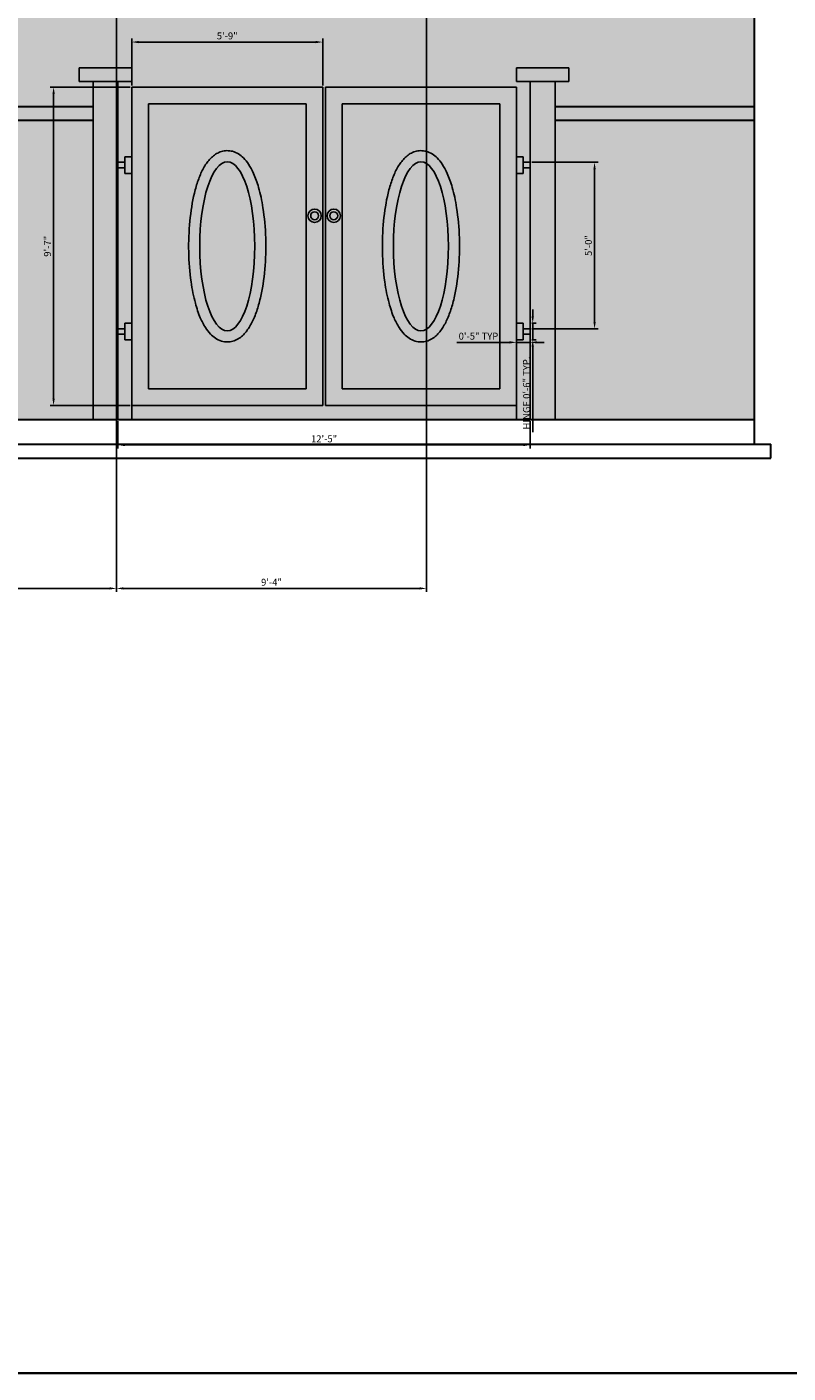
# Model space of a CAD drawing. Units: inches. Extents: x 2391 to 16591, y 7259 to 10239.
# Tile 2 of 27: x 2666 to 2941, y 7259 to 7745. Entities that reach past the tile are written whole.
import ezdxf

# ---------------------------------------------------------------- set-up
doc = ezdxf.new("R2010")
doc.units = ezdxf.units.IN
for name, color, linetype, lineweight in [('A-ANNO-DIMS', 4, 'Continuous', 18), ('A-ANNO-TTLB', 7, 'Continuous', 35), ('A-ELEV', 7, 'Continuous', 30), ('A-ELEV-GATE', 7, 'Continuous', 25), ('A-ELEV-GATE-PATT', 252, 'Continuous', 13), ('A-ELEV-PATT', 8, 'Continuous', 13), ('A-ELEV-SURF-PATT', 253, 'Continuous', 13)]:
    doc.layers.add(name, color=color, linetype=linetype, lineweight=lineweight)
doc.styles.get("Standard").update_dxf_attribs({"font": 'arial.ttf'})
doc.dimstyles.new('ISO-25', dxfattribs={"dimtxt": 2.5, "dimasz": 2.5, "dimexe": 1.25, "dimexo": 0.625, "dimtad": 1, "dimdec": 0, "dimlunit": 3, "dimtxsty": 'Standard', "dimcen": 2.5, "dimadec": 0, "dimazin": 0, "dimtfac": 1, "dimtdec": 0, "dimtmove": 0, "dimatfit": 3, "dimfxl": 1, "dimarcsym": 0})

# ---------------------------------------------------------------- blocks, each defined once
blk = doc.blocks.new('GATE-HINGE-ELEV')
for p, q in [((5, 6), (2.5, 6)), ((2.5, 6), (2.5, 0)), ((2.5, 4), (0, 4)), ((2.5, 2), (0, 2)), ((5, 0), (2.5, 0))]:
    blk.add_line(p, q)
blk = doc.blocks.new('*D63')
at = {"layer": 'A-ANNO-DIMS', "color": 0, "lineweight": -2, "transparency": 16777216}
for p, q in [((2849.16, 7640.15), (2849.16, 7642.65)), ((2848.89, 7637.65), (2850.41, 7637.65)), ((2849.16, 7637.65), (2849.16, 7631.65)), ((2848.89, 7631.65), (2850.41, 7631.65)), ((2849.16, 7629.15), (2849.16, 7598.26))]:
    blk.add_line(p, q, dxfattribs=at)
at = {"layer": 'A-ANNO-DIMS', "color": 0, "transparency": 16777216}
for points in [[(2848.75, 7640.15), (2849.58, 7640.15), (2849.16, 7637.65)], [(2848.75, 7629.15), (2849.58, 7629.15), (2849.16, 7631.65)]]:
    blk.add_solid(points, dxfattribs=at)
at = {"layer": 'Defpoints', "color": 0, "transparency": 16777216}
for p in [(2848.26, 7637.65), (2848.26, 7631.65), (2849.16, 7631.65)]:
    blk.add_point(p, dxfattribs=at)
at = {"layer": 'A-ANNO-DIMS', "color": 0, "transparency": 16777216, "insert": (2847.24, 7612.45), "char_height": 2.5, "attachment_point": 5, "rotation": 90}
blk.add_mtext('HINGE 0\'-6" TYP.', dxfattribs=at)
blk = doc.blocks.new('*D64')
at = {"layer": 'A-ANNO-DIMS', "color": 0, "lineweight": -2, "transparency": 16777216}
for p, q in [((2840.76, 7630.75), (2821.77, 7630.75)), ((2843.26, 7631.02), (2843.26, 7629.5)), ((2848.26, 7630.75), (2843.26, 7630.75)), ((2848.26, 7631.02), (2848.26, 7629.5)), ((2850.76, 7630.75), (2853.26, 7630.75))]:
    blk.add_line(p, q, dxfattribs=at)
at = {"layer": 'A-ANNO-DIMS', "color": 0, "transparency": 16777216}
for points in [[(2840.76, 7631.16), (2840.76, 7630.33), (2843.26, 7630.75)], [(2850.76, 7631.16), (2850.76, 7630.33), (2848.26, 7630.75)]]:
    blk.add_solid(points, dxfattribs=at)
at = {"layer": 'Defpoints', "color": 0, "transparency": 16777216}
for p in [(2843.26, 7631.65), (2843.26, 7630.75), (2848.26, 7631.65)]:
    blk.add_point(p, dxfattribs=at)
at = {"layer": 'A-ANNO-DIMS', "color": 0, "transparency": 16777216, "insert": (2830.02, 7632.65), "char_height": 2.5, "attachment_point": 5}
blk.add_mtext('0\'-5" TYP.', dxfattribs=at)
blk = doc.blocks.new('*D79')
at = {"layer": 'A-ANNO-DIMS', "color": 0, "lineweight": -2, "transparency": 16777216}
for p, q in [((2707.14, 8351.94), (2436.96, 8351.94)), ((2438.21, 7591.44), (2438.21, 8349.44)), ((2490.64, 7588.94), (2436.96, 7588.94))]:
    blk.add_line(p, q, dxfattribs=at)
at = {"layer": 'A-ANNO-DIMS', "color": 0, "transparency": 16777216}
for points in [[(2437.8, 8349.44), (2438.63, 8349.44), (2438.21, 8351.94)], [(2437.8, 7591.44), (2438.63, 7591.44), (2438.21, 7588.94)]]:
    blk.add_solid(points, dxfattribs=at)
at = {"layer": 'Defpoints', "color": 0, "transparency": 16777216}
for p in [(2438.21, 8351.94), (2707.76, 8351.94), (2491.26, 7588.94)]:
    blk.add_point(p, dxfattribs=at)
at = {"layer": 'A-ANNO-DIMS', "color": 0, "transparency": 16777216, "insert": (2436.31, 7970.44), "char_height": 2.5, "attachment_point": 5, "rotation": 90}
blk.add_mtext('63\'-7"', dxfattribs=at)
blk = doc.blocks.new('*D80')
at = {"layer": 'A-ANNO-DIMS', "color": 0, "lineweight": -2, "transparency": 16777216}
for p, q in [((2698.76, 7764.31), (2698.76, 7540.64)), ((2497.26, 7758.31), (2497.26, 7540.64)), ((2499.76, 7541.89), (2696.26, 7541.89))]:
    blk.add_line(p, q, dxfattribs=at)
at = {"layer": 'A-ANNO-DIMS', "color": 0, "transparency": 16777216}
for points in [[(2499.76, 7542.3), (2499.76, 7541.47), (2497.26, 7541.89)], [(2696.26, 7542.3), (2696.26, 7541.47), (2698.76, 7541.89)]]:
    blk.add_solid(points, dxfattribs=at)
at = {"layer": 'Defpoints', "color": 0, "transparency": 16777216}
for p in [(2698.76, 7764.94), (2497.26, 7758.94), (2698.76, 7541.89)]:
    blk.add_point(p, dxfattribs=at)
at = {"layer": 'A-ANNO-DIMS', "color": 0, "transparency": 16777216, "insert": (2598.01, 7543.8), "char_height": 2.5, "attachment_point": 5}
blk.add_mtext('16\'-9 1/2"', dxfattribs=at)
blk = doc.blocks.new('*D81')
at = {"layer": 'A-ANNO-DIMS', "color": 0, "lineweight": -2, "transparency": 16777216}
for p, q in [((2698.76, 7764.31), (2698.76, 7540.64)), ((2810.76, 7764.31), (2810.76, 7540.64)), ((2701.26, 7541.89), (2808.26, 7541.89))]:
    blk.add_line(p, q, dxfattribs=at)
at = {"layer": 'A-ANNO-DIMS', "color": 0, "transparency": 16777216}
for points in [[(2701.26, 7542.3), (2701.26, 7541.47), (2698.76, 7541.89)], [(2808.26, 7542.3), (2808.26, 7541.47), (2810.76, 7541.89)]]:
    blk.add_solid(points, dxfattribs=at)
at = {"layer": 'Defpoints', "color": 0, "transparency": 16777216}
for p in [(2698.76, 7764.94), (2810.76, 7764.94), (2810.76, 7541.89)]:
    blk.add_point(p, dxfattribs=at)
at = {"layer": 'A-ANNO-DIMS', "color": 0, "transparency": 16777216, "insert": (2754.76, 7543.79), "char_height": 2.5, "attachment_point": 5}
blk.add_mtext('9\'-4"', dxfattribs=at)
blk = doc.blocks.new('*D98')
at = {"layer": 'A-ANNO-DIMS', "color": 0, "lineweight": -2, "transparency": 16777216}
for p, q in [((2704.26, 7723.56), (2704.26, 7740.44)), ((2706.76, 7739.19), (2770.76, 7739.19)), ((2773.26, 7723.56), (2773.26, 7740.44))]:
    blk.add_line(p, q, dxfattribs=at)
at = {"layer": 'A-ANNO-DIMS', "color": 0, "transparency": 16777216}
for points in [[(2706.76, 7739.6), (2706.76, 7738.77), (2704.26, 7739.19)], [(2770.76, 7739.6), (2770.76, 7738.77), (2773.26, 7739.19)]]:
    blk.add_solid(points, dxfattribs=at)
at = {"layer": 'Defpoints', "color": 0, "transparency": 16777216}
for p in [(2773.26, 7739.19), (2704.26, 7722.94), (2773.26, 7722.94)]:
    blk.add_point(p, dxfattribs=at)
at = {"layer": 'A-ANNO-DIMS', "color": 0, "transparency": 16777216, "insert": (2738.76, 7741.09), "char_height": 2.5, "attachment_point": 5}
blk.add_mtext('5\'-9"', dxfattribs=at)
blk = doc.blocks.new('*D99')
at = {"layer": 'A-ANNO-DIMS', "color": 0, "lineweight": -2, "transparency": 16777216}
for p, q in [((2703.64, 7722.94), (2674.76, 7722.94)), ((2676.01, 7610.44), (2676.01, 7720.44)), ((2703.64, 7607.94), (2674.76, 7607.94))]:
    blk.add_line(p, q, dxfattribs=at)
at = {"layer": 'A-ANNO-DIMS', "color": 0, "transparency": 16777216}
for points in [[(2675.6, 7720.44), (2676.43, 7720.44), (2676.01, 7722.94)], [(2675.6, 7610.44), (2676.43, 7610.44), (2676.01, 7607.94)]]:
    blk.add_solid(points, dxfattribs=at)
at = {"layer": 'Defpoints', "color": 0, "transparency": 16777216}
for p in [(2676.01, 7722.94), (2704.26, 7722.94), (2704.26, 7607.94)]:
    blk.add_point(p, dxfattribs=at)
at = {"layer": 'A-ANNO-DIMS', "color": 0, "transparency": 16777216, "insert": (2674.11, 7665.44), "char_height": 2.5, "attachment_point": 5, "rotation": 90}
blk.add_mtext('9\'-7"', dxfattribs=at)
blk = doc.blocks.new('*D100')
at = {"layer": 'A-ANNO-DIMS', "color": 0, "lineweight": -2, "transparency": 16777216}
for p, q in [((2699.26, 7602.31), (2699.26, 7592.44)), ((2848.26, 7602.31), (2848.26, 7592.44)), ((2701.76, 7593.69), (2845.76, 7593.69))]:
    blk.add_line(p, q, dxfattribs=at)
at = {"layer": 'A-ANNO-DIMS', "color": 0, "transparency": 16777216}
for points in [[(2701.76, 7594.1), (2701.76, 7593.27), (2699.26, 7593.69)], [(2845.76, 7594.1), (2845.76, 7593.27), (2848.26, 7593.69)]]:
    blk.add_solid(points, dxfattribs=at)
at = {"layer": 'Defpoints', "color": 0, "transparency": 16777216}
for p in [(2699.26, 7602.94), (2848.26, 7602.94), (2848.26, 7593.69)]:
    blk.add_point(p, dxfattribs=at)
at = {"layer": 'A-ANNO-DIMS', "color": 0, "transparency": 16777216, "insert": (2773.76, 7595.59), "char_height": 2.5, "attachment_point": 5}
blk.add_mtext('12\'-5"', dxfattribs=at)
blk = doc.blocks.new('*D101')
at = {"layer": 'A-ANNO-DIMS', "color": 0, "lineweight": -2, "transparency": 16777216}
for p, q in [((2848.89, 7695.78), (2872.76, 7695.78)), ((2871.51, 7638.15), (2871.51, 7693.28)), ((2848.89, 7635.65), (2872.76, 7635.65))]:
    blk.add_line(p, q, dxfattribs=at)
at = {"layer": 'A-ANNO-DIMS', "color": 0, "transparency": 16777216}
for points in [[(2871.1, 7693.28), (2871.93, 7693.28), (2871.51, 7695.78)], [(2871.1, 7638.15), (2871.93, 7638.15), (2871.51, 7635.65)]]:
    blk.add_solid(points, dxfattribs=at)
at = {"layer": 'Defpoints', "color": 0, "transparency": 16777216}
for p in [(2848.26, 7695.78), (2871.51, 7695.78), (2848.26, 7635.65)]:
    blk.add_point(p, dxfattribs=at)
at = {"layer": 'A-ANNO-DIMS', "color": 0, "transparency": 16777216, "insert": (2869.61, 7665.71), "char_height": 2.5, "attachment_point": 5, "rotation": 90}
blk.add_mtext('5\'-0"', dxfattribs=at)

msp = doc.modelspace()

# ---------------------------------------------------------------- hatches: boundary and pattern name
at = {"layer": 'A-ELEV-GATE-PATT'}
h = msp.add_hatch(color=256, dxfattribs=at)
h.dxf.hatch_style = 1
h.paths.add_polyline_path([(2690.26, 7602.94), (2699.26, 7602.94), (2699.26, 7724.94), (2690.26, 7724.94)])
h.paths.add_polyline_path([(2857.26, 7724.94), (2848.26, 7724.94), (2848.26, 7602.94), (2857.26, 7602.94)])
h = msp.add_hatch(color=256, dxfattribs=at)
h.dxf.hatch_style = 1
h.paths.add_polyline_path([(2704.26, 7607.94), (2773.26, 7607.94), (2773.26, 7722.94), (2704.26, 7722.94)])
h.paths.add_polyline_path([(2710.26, 7716.94), (2767.26, 7716.94), (2767.26, 7613.94), (2710.26, 7613.94)], flags=16)
edge = h.paths.add_edge_path(flags=0)
edge.add_spline(control_points=[(2738.76, 7630.9), (2739.47, 7630.9), (2740.17, 7631), (2741.49, 7631.39), (2742.11, 7631.67), (2743.25, 7632.34), (2743.77, 7632.73), (2744.72, 7633.59), (2745.15, 7634.06), (2746.37, 7635.56), (2747.07, 7636.68), (2748.34, 7639.18), (2748.9, 7640.55), (2749.91, 7643.51), (2750.36, 7645.1), (2751.49, 7649.96), (2752.03, 7653.47), (2752.67, 7660.81), (2752.78, 7664.63), (2752.55, 7672.17), (2752.21, 7675.88), (2751.26, 7681.94), (2750.73, 7684.4), (2749.56, 7688.49), (2748.96, 7690.19), (2747.73, 7692.95), (2747.13, 7694.08), (2745.91, 7695.91), (2745.31, 7696.67), (2744.09, 7697.88), (2743.5, 7698.36), (2742.17, 7699.19), (2741.43, 7699.52), (2739.99, 7699.9), (2739.31, 7699.99), (2737.96, 7699.96), (2737.29, 7699.85), (2736.03, 7699.48), (2735.44, 7699.21), (2734.35, 7698.58), (2733.85, 7698.21), (2732.92, 7697.39), (2732.5, 7696.95), (2731.29, 7695.51), (2730.59, 7694.42), (2729.33, 7692), (2728.77, 7690.67), (2727.75, 7687.8), (2727.29, 7686.25), (2726.15, 7681.52), (2725.6, 7678.1), (2724.9, 7670.92), (2724.76, 7667.17), (2724.92, 7659.73), (2725.2, 7656.05), (2726.09, 7649.88), (2726.6, 7647.3), (2727.76, 7643.01), (2728.35, 7641.24), (2729.58, 7638.34), (2730.18, 7637.17), (2731.41, 7635.24), (2732, 7634.45), (2733.22, 7633.18), (2733.82, 7632.67), (2735.15, 7631.79), (2735.9, 7631.43), (2737.36, 7631), (2738.06, 7630.9), (2738.76, 7630.9)], knot_values=[0, 0, 0, 0, 0.095196, 0.095196, 0.190392, 0.190392, 0.285588, 0.285588, 0.380784, 0.380784, 0.570897, 0.570897, 0.76101, 0.76101, 0.951123, 0.951123, 1.307609, 1.307609, 1.664096, 1.664096, 2.020583, 2.020583, 2.290036, 2.290036, 2.5108, 2.5108, 2.687191, 2.687191, 2.829292, 2.829292, 2.942747, 2.942747, 3.056202, 3.056202, 3.147245, 3.147245, 3.238288, 3.238288, 3.329331, 3.329331, 3.420374, 3.420374, 3.511418, 3.511418, 3.698581, 3.698581, 3.885745, 3.885745, 4.072908, 4.072908, 4.42383, 4.42383, 4.774752, 4.774752, 5.125674, 5.125674, 5.403289, 5.403289, 5.629501, 5.629501, 5.810378, 5.810378, 5.956164, 5.956164, 6.072402, 6.072402, 6.18864, 6.18864, 6.283185, 6.283185, 6.283185, 6.283185], degree=3, periodic=0)
edge = h.paths.add_edge_path(flags=0)
edge.add_ellipse((2738.76, 7665.44), major_axis=(0, -30.54), ratio=0.325581, start_angle=0, end_angle=360)
h.paths.add_polyline_path([(2771.76, 7676.46, -1), (2768.92, 7676.46, -1)], flags=16)
h.paths.add_polyline_path([(2774.26, 7607.94), (2843.26, 7607.94), (2843.26, 7722.94), (2774.26, 7722.94)])
h.paths.add_polyline_path([(2780.26, 7716.94), (2837.26, 7716.94), (2837.26, 7613.94), (2780.26, 7613.94)], flags=16)
edge = h.paths.add_edge_path(flags=0)
edge.add_spline(control_points=[(2808.76, 7630.9), (2809.47, 7630.9), (2810.17, 7631), (2811.49, 7631.39), (2812.11, 7631.67), (2813.25, 7632.34), (2813.77, 7632.73), (2814.72, 7633.59), (2815.15, 7634.06), (2816.37, 7635.56), (2817.07, 7636.68), (2818.34, 7639.18), (2818.9, 7640.55), (2819.91, 7643.51), (2820.36, 7645.1), (2821.49, 7649.96), (2822.03, 7653.47), (2822.67, 7660.81), (2822.78, 7664.63), (2822.55, 7672.17), (2822.21, 7675.88), (2821.26, 7681.94), (2820.73, 7684.4), (2819.56, 7688.49), (2818.96, 7690.19), (2817.73, 7692.95), (2817.13, 7694.08), (2815.91, 7695.91), (2815.31, 7696.67), (2814.09, 7697.88), (2813.5, 7698.36), (2812.17, 7699.19), (2811.43, 7699.52), (2809.99, 7699.9), (2809.31, 7699.99), (2807.96, 7699.96), (2807.29, 7699.85), (2806.03, 7699.48), (2805.44, 7699.21), (2804.35, 7698.58), (2803.85, 7698.21), (2802.92, 7697.39), (2802.5, 7696.95), (2801.29, 7695.51), (2800.59, 7694.42), (2799.33, 7692), (2798.77, 7690.67), (2797.75, 7687.8), (2797.29, 7686.25), (2796.15, 7681.52), (2795.6, 7678.1), (2794.9, 7670.92), (2794.76, 7667.17), (2794.92, 7659.73), (2795.2, 7656.05), (2796.09, 7649.88), (2796.6, 7647.3), (2797.76, 7643.01), (2798.35, 7641.24), (2799.58, 7638.34), (2800.18, 7637.17), (2801.41, 7635.24), (2802, 7634.45), (2803.22, 7633.18), (2803.82, 7632.67), (2805.15, 7631.79), (2805.9, 7631.43), (2807.36, 7631), (2808.06, 7630.9), (2808.76, 7630.9)], knot_values=[0, 0, 0, 0, 0.095196, 0.095196, 0.190392, 0.190392, 0.285588, 0.285588, 0.380784, 0.380784, 0.570897, 0.570897, 0.76101, 0.76101, 0.951123, 0.951123, 1.307609, 1.307609, 1.664096, 1.664096, 2.020583, 2.020583, 2.290036, 2.290036, 2.5108, 2.5108, 2.687191, 2.687191, 2.829292, 2.829292, 2.942747, 2.942747, 3.056202, 3.056202, 3.147245, 3.147245, 3.238288, 3.238288, 3.329331, 3.329331, 3.420374, 3.420374, 3.511418, 3.511418, 3.698581, 3.698581, 3.885745, 3.885745, 4.072908, 4.072908, 4.42383, 4.42383, 4.774752, 4.774752, 5.125674, 5.125674, 5.403289, 5.403289, 5.629501, 5.629501, 5.810378, 5.810378, 5.956164, 5.956164, 6.072402, 6.072402, 6.18864, 6.18864, 6.283185, 6.283185, 6.283185, 6.283185], degree=3, periodic=0)
edge = h.paths.add_edge_path(flags=0)
edge.add_ellipse((2808.76, 7665.44), major_axis=(0, -30.54), ratio=0.325581, start_angle=0, end_angle=360)
h.paths.add_polyline_path([(2779.68, 7676.46, -1), (2774.84, 7676.46, -1)], flags=16)
h.paths.add_polyline_path([(2778.68, 7676.46, -1), (2775.84, 7676.46, -1)], flags=0)
h = msp.add_hatch(color=256, dxfattribs=at)
h.dxf.hatch_style = 1
h.paths.add_polyline_path([(2710.26, 7716.94), (2710.26, 7613.94), (2767.26, 7613.94), (2767.26, 7716.94)])
edge = h.paths.add_edge_path(flags=16)
edge.add_spline(control_points=[(2738.76, 7630.9), (2739.47, 7630.9), (2740.17, 7631), (2741.49, 7631.39), (2742.11, 7631.67), (2743.25, 7632.34), (2743.77, 7632.73), (2744.72, 7633.59), (2745.15, 7634.06), (2746.37, 7635.56), (2747.07, 7636.68), (2748.34, 7639.18), (2748.9, 7640.55), (2749.91, 7643.51), (2750.36, 7645.1), (2751.49, 7649.96), (2752.03, 7653.47), (2752.67, 7660.81), (2752.78, 7664.63), (2752.55, 7672.17), (2752.21, 7675.88), (2751.26, 7681.94), (2750.73, 7684.4), (2749.56, 7688.49), (2748.96, 7690.19), (2747.73, 7692.95), (2747.13, 7694.08), (2745.91, 7695.91), (2745.31, 7696.67), (2744.09, 7697.88), (2743.5, 7698.36), (2742.17, 7699.19), (2741.43, 7699.52), (2739.99, 7699.9), (2739.31, 7699.99), (2737.96, 7699.96), (2737.29, 7699.85), (2736.03, 7699.48), (2735.44, 7699.21), (2734.35, 7698.58), (2733.85, 7698.21), (2732.92, 7697.39), (2732.5, 7696.95), (2731.29, 7695.51), (2730.59, 7694.42), (2729.33, 7692), (2728.77, 7690.67), (2727.75, 7687.8), (2727.29, 7686.25), (2726.15, 7681.52), (2725.6, 7678.1), (2724.9, 7670.92), (2724.76, 7667.17), (2724.92, 7659.73), (2725.2, 7656.05), (2726.09, 7649.88), (2726.6, 7647.3), (2727.76, 7643.01), (2728.35, 7641.24), (2729.58, 7638.34), (2730.18, 7637.17), (2731.41, 7635.24), (2732, 7634.45), (2733.22, 7633.18), (2733.82, 7632.67), (2735.15, 7631.79), (2735.9, 7631.43), (2737.36, 7631), (2738.06, 7630.9), (2738.76, 7630.9)], knot_values=[0, 0, 0, 0, 0.095196, 0.095196, 0.190392, 0.190392, 0.285588, 0.285588, 0.380784, 0.380784, 0.570897, 0.570897, 0.76101, 0.76101, 0.951123, 0.951123, 1.307609, 1.307609, 1.664096, 1.664096, 2.020583, 2.020583, 2.290036, 2.290036, 2.5108, 2.5108, 2.687191, 2.687191, 2.829292, 2.829292, 2.942747, 2.942747, 3.056202, 3.056202, 3.147245, 3.147245, 3.238288, 3.238288, 3.329331, 3.329331, 3.420374, 3.420374, 3.511418, 3.511418, 3.698581, 3.698581, 3.885745, 3.885745, 4.072908, 4.072908, 4.42383, 4.42383, 4.774752, 4.774752, 5.125674, 5.125674, 5.403289, 5.403289, 5.629501, 5.629501, 5.810378, 5.810378, 5.956164, 5.956164, 6.072402, 6.072402, 6.18864, 6.18864, 6.283185, 6.283185, 6.283185, 6.283185], degree=3, periodic=0)
edge = h.paths.add_edge_path(flags=0)
edge.add_ellipse((2738.76, 7665.44), major_axis=(0, -30.54), ratio=0.325581, start_angle=0, end_angle=360)
h.paths.add_polyline_path([(2780.26, 7716.94), (2780.26, 7613.94), (2837.26, 7613.94), (2837.26, 7716.94)])
edge = h.paths.add_edge_path(flags=16)
edge.add_spline(control_points=[(2808.76, 7630.9), (2809.47, 7630.9), (2810.17, 7631), (2811.49, 7631.39), (2812.11, 7631.67), (2813.25, 7632.34), (2813.77, 7632.73), (2814.72, 7633.59), (2815.15, 7634.06), (2816.37, 7635.56), (2817.07, 7636.68), (2818.34, 7639.18), (2818.9, 7640.55), (2819.91, 7643.51), (2820.36, 7645.1), (2821.49, 7649.96), (2822.03, 7653.47), (2822.67, 7660.81), (2822.78, 7664.63), (2822.55, 7672.17), (2822.21, 7675.88), (2821.26, 7681.94), (2820.73, 7684.4), (2819.56, 7688.49), (2818.96, 7690.19), (2817.73, 7692.95), (2817.13, 7694.08), (2815.91, 7695.91), (2815.31, 7696.67), (2814.09, 7697.88), (2813.5, 7698.36), (2812.17, 7699.19), (2811.43, 7699.52), (2809.99, 7699.9), (2809.31, 7699.99), (2807.96, 7699.96), (2807.29, 7699.85), (2806.03, 7699.48), (2805.44, 7699.21), (2804.35, 7698.58), (2803.85, 7698.21), (2802.92, 7697.39), (2802.5, 7696.95), (2801.29, 7695.51), (2800.59, 7694.42), (2799.33, 7692), (2798.77, 7690.67), (2797.75, 7687.8), (2797.29, 7686.25), (2796.15, 7681.52), (2795.6, 7678.1), (2794.9, 7670.92), (2794.76, 7667.17), (2794.92, 7659.73), (2795.2, 7656.05), (2796.09, 7649.88), (2796.6, 7647.3), (2797.76, 7643.01), (2798.35, 7641.24), (2799.58, 7638.34), (2800.18, 7637.17), (2801.41, 7635.24), (2802, 7634.45), (2803.22, 7633.18), (2803.82, 7632.67), (2805.15, 7631.79), (2805.9, 7631.43), (2807.36, 7631), (2808.06, 7630.9), (2808.76, 7630.9)], knot_values=[0, 0, 0, 0, 0.095196, 0.095196, 0.190392, 0.190392, 0.285588, 0.285588, 0.380784, 0.380784, 0.570897, 0.570897, 0.76101, 0.76101, 0.951123, 0.951123, 1.307609, 1.307609, 1.664096, 1.664096, 2.020583, 2.020583, 2.290036, 2.290036, 2.5108, 2.5108, 2.687191, 2.687191, 2.829292, 2.829292, 2.942747, 2.942747, 3.056202, 3.056202, 3.147245, 3.147245, 3.238288, 3.238288, 3.329331, 3.329331, 3.420374, 3.420374, 3.511418, 3.511418, 3.698581, 3.698581, 3.885745, 3.885745, 4.072908, 4.072908, 4.42383, 4.42383, 4.774752, 4.774752, 5.125674, 5.125674, 5.403289, 5.403289, 5.629501, 5.629501, 5.810378, 5.810378, 5.956164, 5.956164, 6.072402, 6.072402, 6.18864, 6.18864, 6.283185, 6.283185, 6.283185, 6.283185], degree=3, periodic=0)
edge = h.paths.add_edge_path(flags=0)
edge.add_ellipse((2808.76, 7665.44), major_axis=(0, -30.54), ratio=0.325581, start_angle=0, end_angle=360)
h = msp.add_hatch(color=256, dxfattribs=at)
h.dxf.hatch_style = 1
h.paths.add_polyline_path([(2704.26, 7697.78), (2701.76, 7697.78), (2701.76, 7691.78), (2704.26, 7691.78)])
h.paths.add_polyline_path([(2701.76, 7695.78), (2699.26, 7695.78), (2699.26, 7693.78), (2701.76, 7693.78)])
h.paths.add_polyline_path([(2701.76, 7635.65), (2699.26, 7635.65), (2699.26, 7633.65), (2701.76, 7633.65)])
h.paths.add_polyline_path([(2704.26, 7637.65), (2701.76, 7637.65), (2701.76, 7631.65), (2704.26, 7631.65)])
h.paths.add_polyline_path([(2848.26, 7695.78), (2845.76, 7695.78), (2845.76, 7693.78), (2848.26, 7693.78)])
h.paths.add_polyline_path([(2845.76, 7697.78), (2843.26, 7697.78), (2843.26, 7691.78), (2845.76, 7691.78)])
h.paths.add_polyline_path([(2845.76, 7637.65), (2843.26, 7637.65), (2843.26, 7631.65), (2845.76, 7631.65)])
h.paths.add_polyline_path([(2848.26, 7635.65), (2845.76, 7635.65), (2845.76, 7633.65), (2848.26, 7633.65)])
h = msp.add_hatch(color=256, dxfattribs=at)
h.dxf.hatch_style = 1
edge = h.paths.add_edge_path()
edge.add_spline(control_points=[(2738.76, 7630.9), (2739.47, 7630.9), (2740.17, 7631), (2741.49, 7631.39), (2742.11, 7631.67), (2743.25, 7632.34), (2743.77, 7632.73), (2744.72, 7633.59), (2745.15, 7634.06), (2746.37, 7635.56), (2747.07, 7636.68), (2748.34, 7639.18), (2748.9, 7640.55), (2749.91, 7643.51), (2750.36, 7645.1), (2751.49, 7649.96), (2752.03, 7653.47), (2752.67, 7660.81), (2752.78, 7664.63), (2752.55, 7672.17), (2752.21, 7675.88), (2751.26, 7681.94), (2750.73, 7684.4), (2749.56, 7688.49), (2748.96, 7690.19), (2747.73, 7692.95), (2747.13, 7694.08), (2745.91, 7695.91), (2745.31, 7696.67), (2744.09, 7697.88), (2743.5, 7698.36), (2742.17, 7699.19), (2741.43, 7699.52), (2739.99, 7699.9), (2739.31, 7699.99), (2737.96, 7699.96), (2737.29, 7699.85), (2736.03, 7699.48), (2735.44, 7699.21), (2734.35, 7698.58), (2733.85, 7698.21), (2732.92, 7697.39), (2732.5, 7696.95), (2731.29, 7695.51), (2730.59, 7694.42), (2729.33, 7692), (2728.77, 7690.67), (2727.75, 7687.8), (2727.29, 7686.25), (2726.15, 7681.52), (2725.6, 7678.1), (2724.9, 7670.92), (2724.76, 7667.17), (2724.92, 7659.73), (2725.2, 7656.05), (2726.09, 7649.88), (2726.6, 7647.3), (2727.76, 7643.01), (2728.35, 7641.24), (2729.58, 7638.34), (2730.18, 7637.17), (2731.41, 7635.24), (2732, 7634.45), (2733.22, 7633.18), (2733.82, 7632.67), (2735.15, 7631.79), (2735.9, 7631.43), (2737.36, 7631), (2738.06, 7630.9), (2738.76, 7630.9)], knot_values=[0, 0, 0, 0, 0.095196, 0.095196, 0.190392, 0.190392, 0.285588, 0.285588, 0.380784, 0.380784, 0.570897, 0.570897, 0.76101, 0.76101, 0.951123, 0.951123, 1.307609, 1.307609, 1.664096, 1.664096, 2.020583, 2.020583, 2.290036, 2.290036, 2.5108, 2.5108, 2.687191, 2.687191, 2.829292, 2.829292, 2.942747, 2.942747, 3.056202, 3.056202, 3.147245, 3.147245, 3.238288, 3.238288, 3.329331, 3.329331, 3.420374, 3.420374, 3.511418, 3.511418, 3.698581, 3.698581, 3.885745, 3.885745, 4.072908, 4.072908, 4.42383, 4.42383, 4.774752, 4.774752, 5.125674, 5.125674, 5.403289, 5.403289, 5.629501, 5.629501, 5.810378, 5.810378, 5.956164, 5.956164, 6.072402, 6.072402, 6.18864, 6.18864, 6.283185, 6.283185, 6.283185, 6.283185], degree=3, periodic=0)
edge = h.paths.add_edge_path(flags=16)
edge.add_ellipse((2738.76, 7665.44), major_axis=(0, -30.54), ratio=0.325581, start_angle=0, end_angle=360)
edge = h.paths.add_edge_path()
edge.add_spline(control_points=[(2808.76, 7630.9), (2809.47, 7630.9), (2810.17, 7631), (2811.49, 7631.39), (2812.11, 7631.67), (2813.25, 7632.34), (2813.77, 7632.73), (2814.72, 7633.59), (2815.15, 7634.06), (2816.37, 7635.56), (2817.07, 7636.68), (2818.34, 7639.18), (2818.9, 7640.55), (2819.91, 7643.51), (2820.36, 7645.1), (2821.49, 7649.96), (2822.03, 7653.47), (2822.67, 7660.81), (2822.78, 7664.63), (2822.55, 7672.17), (2822.21, 7675.88), (2821.26, 7681.94), (2820.73, 7684.4), (2819.56, 7688.49), (2818.96, 7690.19), (2817.73, 7692.95), (2817.13, 7694.08), (2815.91, 7695.91), (2815.31, 7696.67), (2814.09, 7697.88), (2813.5, 7698.36), (2812.17, 7699.19), (2811.43, 7699.52), (2809.99, 7699.9), (2809.31, 7699.99), (2807.96, 7699.96), (2807.29, 7699.85), (2806.03, 7699.48), (2805.44, 7699.21), (2804.35, 7698.58), (2803.85, 7698.21), (2802.92, 7697.39), (2802.5, 7696.95), (2801.29, 7695.51), (2800.59, 7694.42), (2799.33, 7692), (2798.77, 7690.67), (2797.75, 7687.8), (2797.29, 7686.25), (2796.15, 7681.52), (2795.6, 7678.1), (2794.9, 7670.92), (2794.76, 7667.17), (2794.92, 7659.73), (2795.2, 7656.05), (2796.09, 7649.88), (2796.6, 7647.3), (2797.76, 7643.01), (2798.35, 7641.24), (2799.58, 7638.34), (2800.18, 7637.17), (2801.41, 7635.24), (2802, 7634.45), (2803.22, 7633.18), (2803.82, 7632.67), (2805.15, 7631.79), (2805.9, 7631.43), (2807.36, 7631), (2808.06, 7630.9), (2808.76, 7630.9)], knot_values=[0, 0, 0, 0, 0.095196, 0.095196, 0.190392, 0.190392, 0.285588, 0.285588, 0.380784, 0.380784, 0.570897, 0.570897, 0.76101, 0.76101, 0.951123, 0.951123, 1.307609, 1.307609, 1.664096, 1.664096, 2.020583, 2.020583, 2.290036, 2.290036, 2.5108, 2.5108, 2.687191, 2.687191, 2.829292, 2.829292, 2.942747, 2.942747, 3.056202, 3.056202, 3.147245, 3.147245, 3.238288, 3.238288, 3.329331, 3.329331, 3.420374, 3.420374, 3.511418, 3.511418, 3.698581, 3.698581, 3.885745, 3.885745, 4.072908, 4.072908, 4.42383, 4.42383, 4.774752, 4.774752, 5.125674, 5.125674, 5.403289, 5.403289, 5.629501, 5.629501, 5.810378, 5.810378, 5.956164, 5.956164, 6.072402, 6.072402, 6.18864, 6.18864, 6.283185, 6.283185, 6.283185, 6.283185], degree=3, periodic=0)
edge = h.paths.add_edge_path(flags=16)
edge.add_ellipse((2808.76, 7665.44), major_axis=(0, -30.54), ratio=0.325581, start_angle=0, end_angle=360)
h = msp.add_hatch(color=256, dxfattribs=at)
h.dxf.hatch_style = 1
edge = h.paths.add_edge_path()
edge.add_ellipse((2738.76, 7665.44), major_axis=(0, -30.54), ratio=0.325581, start_angle=0, end_angle=360)
edge = h.paths.add_edge_path()
edge.add_ellipse((2808.76, 7665.44), major_axis=(0, -30.54), ratio=0.325581, start_angle=0, end_angle=360)
h = msp.add_hatch(color=256, dxfattribs=at)
h.dxf.hatch_style = 1
h.paths.add_polyline_path([(2772.76, 7676.46, 1), (2767.92, 7676.46, 1)])
h.paths.add_polyline_path([(2771.76, 7676.46, 1), (2768.92, 7676.46, 1)], flags=16)
h.paths.add_polyline_path([(2779.68, 7676.46, 1), (2774.84, 7676.46, 1)])
h.paths.add_polyline_path([(2778.68, 7676.46, 1), (2775.84, 7676.46, 1)], flags=16)
h = msp.add_hatch(color=256, dxfattribs=at)
h.dxf.hatch_style = 1
h.paths.add_polyline_path([(2771.76, 7676.46, 1), (2768.92, 7676.46, 1)])
h.paths.add_polyline_path([(2778.68, 7676.46, 1), (2775.84, 7676.46, 1)])
at = {"layer": 'A-ELEV-PATT'}
h = msp.add_hatch(dxfattribs=at)
h.set_pattern_fill('GRAVEL', color=256)
h.paths.add_polyline_path([(2690.26, 7602.94), (2690.26, 7710.94), (2497.26, 7710.94), (2497.26, 7602.94)])
h.paths.add_polyline_path([(2929.26, 7710.94), (2857.26, 7710.94), (2857.26, 7602.94), (2929.26, 7602.94)])
at = {"layer": 'A-ELEV-SURF-PATT'}
h = msp.add_hatch(color=256, dxfattribs=at)
h.dxf.hatch_style = 1
h.paths.add_polyline_path([(2929.26, 7758.94), (2497.26, 7758.94), (2497.26, 7715.94), (2690.26, 7715.94), (2690.26, 7724.94), (2685.26, 7724.94), (2685.26, 7729.94), (2704.26, 7729.94), (2704.26, 7724.94), (2699.26, 7724.94), (2699.26, 7695.78), (2701.76, 7695.78), (2701.76, 7697.78), (2704.26, 7697.78), (2704.26, 7722.94), (2773.26, 7722.94), (2773.26, 7607.94), (2704.26, 7607.94), (2704.26, 7602.94), (2843.26, 7602.94), (2843.26, 7607.94), (2774.26, 7607.94), (2774.26, 7722.94), (2843.26, 7722.94), (2843.26, 7697.78), (2845.76, 7697.78), (2845.76, 7695.78), (2848.26, 7695.78), (2848.26, 7724.94), (2843.26, 7724.94), (2843.26, 7729.94), (2862.26, 7729.94), (2862.26, 7724.94), (2857.26, 7724.94), (2857.26, 7715.94), (2929.26, 7715.94)])
h.paths.add_polyline_path([(2848.26, 7693.78), (2845.76, 7693.78), (2845.76, 7691.78), (2843.26, 7691.78), (2843.26, 7637.65), (2845.76, 7637.65), (2845.76, 7635.65), (2848.26, 7635.65)], flags=17)
h.paths.add_polyline_path([(2848.26, 7633.65), (2845.76, 7633.65), (2845.76, 7631.65), (2843.26, 7631.65), (2843.26, 7602.94), (2848.26, 7602.94)], flags=17)
h.paths.add_polyline_path([(2704.26, 7631.65), (2701.76, 7631.65), (2701.76, 7633.65), (2699.26, 7633.65), (2699.26, 7602.94), (2704.26, 7602.94), (2704.26, 7607.94)], flags=17)
h.paths.add_polyline_path([(2704.26, 7691.78), (2701.76, 7691.78), (2701.76, 7693.78), (2699.26, 7693.78), (2699.26, 7635.65), (2701.76, 7635.65), (2701.76, 7637.65), (2704.26, 7637.65)], flags=17)
h = msp.add_hatch(color=256, dxfattribs=at)
h.dxf.hatch_style = 1
h.paths.add_polyline_path([(2690.26, 7715.94), (2497.26, 7715.94), (2497.26, 7710.94), (2690.26, 7710.94)])
h.paths.add_polyline_path([(2704.26, 7729.94), (2685.26, 7729.94), (2685.26, 7724.94), (2704.26, 7724.94)])
h.paths.add_polyline_path([(2862.26, 7729.94), (2843.26, 7729.94), (2843.26, 7724.94), (2862.26, 7724.94)])
h.paths.add_polyline_path([(2929.26, 7715.94), (2857.26, 7715.94), (2857.26, 7710.94), (2929.26, 7710.94)])

# ---------------------------------------------------------------- linework, layer by layer
at = {"layer": 'A-ANNO-TTLB'}
msp.add_lwpolyline([(2391.28, 10239.38), (4154.2, 10239.38), (4154.2, 7258.54), (2391.28, 7258.54)], close=True, dxfattribs=at)
at = {"layer": 'A-ELEV'}
for p, q in [((2929.26, 7593.94), (2929.26, 7758.94)), ((2497.26, 7715.94), (2690.26, 7715.94)), ((2857.26, 7715.94), (2929.26, 7715.94)), ((2497.26, 7710.94), (2690.26, 7710.94)), ((2857.26, 7710.94), (2929.26, 7710.94)), ((2497.26, 7602.94), (2929.26, 7602.94)), ((2491.26, 7593.94), (2935.26, 7593.94)), ((2935.26, 7588.94), (2935.26, 7593.94)), ((2491.26, 7588.94), (2935.26, 7588.94))]:
    msp.add_line(p, q, dxfattribs=at)
at = {"layer": 'A-ELEV-GATE'}
for p, q in [((2704.26, 7729.94), (2685.26, 7729.94)), ((2685.26, 7724.94), (2685.26, 7729.94)), ((2704.26, 7724.94), (2704.26, 7729.94)), ((2843.26, 7729.94), (2862.26, 7729.94)), ((2843.26, 7724.94), (2843.26, 7729.94)), ((2862.26, 7724.94), (2862.26, 7729.94)), ((2704.26, 7724.94), (2685.26, 7724.94)), ((2690.26, 7602.94), (2690.26, 7724.94)), ((2699.26, 7602.94), (2699.26, 7724.94)), ((2843.26, 7724.94), (2862.26, 7724.94)), ((2848.26, 7602.94), (2848.26, 7724.94)), ((2857.26, 7602.94), (2857.26, 7724.94)), ((2704.26, 7602.94), (2704.26, 7722.94)), ((2704.26, 7722.94), (2773.26, 7722.94)), ((2773.26, 7722.94), (2773.26, 7607.94)), ((2774.26, 7722.94), (2774.26, 7607.94)), ((2774.26, 7722.94), (2843.26, 7722.94)), ((2843.26, 7602.94), (2843.26, 7722.94)), ((2710.26, 7716.94), (2767.26, 7716.94)), ((2710.26, 7613.94), (2710.26, 7716.94)), ((2767.26, 7716.94), (2767.26, 7613.94)), ((2780.26, 7716.94), (2780.26, 7613.94)), ((2780.26, 7716.94), (2837.26, 7716.94)), ((2837.26, 7613.94), (2837.26, 7716.94)), ((2710.26, 7613.94), (2767.26, 7613.94)), ((2780.26, 7613.94), (2837.26, 7613.94)), ((2704.26, 7607.94), (2773.26, 7607.94)), ((2774.26, 7607.94), (2843.26, 7607.94))]:
    msp.add_line(p, q, dxfattribs=at)
for centre, radius in [((2770.34, 7676.46), 2.42), ((2770.34, 7676.46), 1.42), ((2777.26, 7676.46), 2.42), ((2777.26, 7676.46), 1.42)]:
    msp.add_circle(centre, radius, dxfattribs=at)
for centre in [(2738.76, 7665.44), (2808.76, 7665.44)]:
    msp.add_ellipse(centre, major_axis=(0, -30.54), ratio=0.325581, dxfattribs=at)
for points in [[(2738.76, 7630.9), (2739.47, 7630.9), (2740.17, 7631), (2741.49, 7631.39), (2742.11, 7631.67), (2743.25, 7632.34), (2743.77, 7632.73), (2744.72, 7633.59), (2745.15, 7634.06), (2746.37, 7635.56), (2747.07, 7636.68), (2748.34, 7639.18), (2748.9, 7640.55), (2749.91, 7643.51), (2750.36, 7645.1), (2751.49, 7649.96), (2752.03, 7653.47), (2752.67, 7660.81), (2752.78, 7664.63), (2752.55, 7672.17), (2752.21, 7675.88), (2751.26, 7681.94), (2750.73, 7684.4), (2749.56, 7688.49), (2748.96, 7690.19), (2747.73, 7692.95), (2747.13, 7694.08), (2745.91, 7695.91), (2745.31, 7696.67), (2744.09, 7697.88), (2743.5, 7698.36), (2742.17, 7699.19), (2741.43, 7699.52), (2739.99, 7699.9), (2739.31, 7699.99), (2737.96, 7699.96), (2737.29, 7699.85), (2736.03, 7699.48), (2735.44, 7699.21), (2734.35, 7698.58), (2733.85, 7698.21), (2732.92, 7697.39), (2732.5, 7696.95), (2731.29, 7695.51), (2730.59, 7694.42), (2729.33, 7692), (2728.77, 7690.67), (2727.75, 7687.8), (2727.29, 7686.25), (2726.15, 7681.52), (2725.6, 7678.1), (2724.9, 7670.92), (2724.76, 7667.17), (2724.92, 7659.73), (2725.2, 7656.05), (2726.09, 7649.88), (2726.6, 7647.3), (2727.76, 7643.01), (2728.35, 7641.24), (2729.58, 7638.34), (2730.18, 7637.17), (2731.41, 7635.24), (2732, 7634.45), (2733.22, 7633.18), (2733.82, 7632.67), (2735.15, 7631.79), (2735.9, 7631.43), (2737.36, 7631), (2738.06, 7630.9), (2738.76, 7630.9)], [(2808.76, 7630.9), (2809.47, 7630.9), (2810.17, 7631), (2811.49, 7631.39), (2812.11, 7631.67), (2813.25, 7632.34), (2813.77, 7632.73), (2814.72, 7633.59), (2815.15, 7634.06), (2816.37, 7635.56), (2817.07, 7636.68), (2818.34, 7639.18), (2818.9, 7640.55), (2819.91, 7643.51), (2820.36, 7645.1), (2821.49, 7649.96), (2822.03, 7653.47), (2822.67, 7660.81), (2822.78, 7664.63), (2822.55, 7672.17), (2822.21, 7675.88), (2821.26, 7681.94), (2820.73, 7684.4), (2819.56, 7688.49), (2818.96, 7690.19), (2817.73, 7692.95), (2817.13, 7694.08), (2815.91, 7695.91), (2815.31, 7696.67), (2814.09, 7697.88), (2813.5, 7698.36), (2812.17, 7699.19), (2811.43, 7699.52), (2809.99, 7699.9), (2809.31, 7699.99), (2807.96, 7699.96), (2807.29, 7699.85), (2806.03, 7699.48), (2805.44, 7699.21), (2804.35, 7698.58), (2803.85, 7698.21), (2802.92, 7697.39), (2802.5, 7696.95), (2801.29, 7695.51), (2800.59, 7694.42), (2799.33, 7692), (2798.77, 7690.67), (2797.75, 7687.8), (2797.29, 7686.25), (2796.15, 7681.52), (2795.6, 7678.1), (2794.9, 7670.92), (2794.76, 7667.17), (2794.92, 7659.73), (2795.2, 7656.05), (2796.09, 7649.88), (2796.6, 7647.3), (2797.76, 7643.01), (2798.35, 7641.24), (2799.58, 7638.34), (2800.18, 7637.17), (2801.41, 7635.24), (2802, 7634.45), (2803.22, 7633.18), (2803.82, 7632.67), (2805.15, 7631.79), (2805.9, 7631.43), (2807.36, 7631), (2808.06, 7630.9), (2808.76, 7630.9)]]:
    msp.add_open_spline(points, degree=3, knots=[0, 0, 0, 0, 0.095196, 0.095196, 0.190392, 0.190392, 0.285588, 0.285588, 0.380784, 0.380784, 0.570897, 0.570897, 0.76101, 0.76101, 0.951123, 0.951123, 1.307609, 1.307609, 1.664096, 1.664096, 2.020583, 2.020583, 2.290036, 2.290036, 2.5108, 2.5108, 2.687191, 2.687191, 2.829292, 2.829292, 2.942747, 2.942747, 3.056202, 3.056202, 3.147245, 3.147245, 3.238288, 3.238288, 3.329331, 3.329331, 3.420374, 3.420374, 3.511418, 3.511418, 3.698581, 3.698581, 3.885745, 3.885745, 4.072908, 4.072908, 4.42383, 4.42383, 4.774752, 4.774752, 5.125674, 5.125674, 5.403289, 5.403289, 5.629501, 5.629501, 5.810378, 5.810378, 5.956164, 5.956164, 6.072402, 6.072402, 6.18864, 6.18864, 6.283185, 6.283185, 6.283185, 6.283185], dxfattribs=at)

# ---------------------------------------------------------------- block references
for p in [(2699.26, 7691.78), (2699.26, 7631.65)]:
    msp.add_blockref('GATE-HINGE-ELEV', p, dxfattribs=at)
at = {"layer": 'A-ELEV-GATE', "rotation": 180}
for p in [(2848.26, 7697.78), (2848.26, 7637.65)]:
    msp.add_blockref('GATE-HINGE-ELEV', p, dxfattribs=at)

# ---------------------------------------------------------------- dimensions: what is measured, and where the dimension line sits
at = {"layer": 'A-ANNO-DIMS'}
for base, p1, p2, picture, middle in [((2438.21, 8351.94), (2491.26, 7588.94), (2707.76, 8351.94), '*D79', (2436.31, 7970.44)), ((2676.01, 7722.94), (2704.26, 7607.94), (2704.26, 7722.94), '*D99', (2674.11, 7665.44)), ((2871.51, 7695.78), (2848.26, 7635.65), (2848.26, 7695.78), '*D101', (2869.61, 7665.71))]:
    dim = msp.add_linear_dim(base=base, p1=p1, p2=p2, angle=90, dimstyle='ISO-25', override={"dimdec": 1, "dimlfac": 1, "dimrnd": 0, "dimzin": 1, "dimdsep": 46, "dimlunit": 4, "dimfrac": 2}, dxfattribs=at)
    dim.commit()
    dim.dimension.update_dxf_attribs({"geometry": picture, "text_midpoint": middle})
for base, p1, p2, picture, middle in [((2698.76, 7541.89), (2497.26, 7758.94), (2698.76, 7764.94), '*D80', (2598.01, 7543.8)), ((2810.76, 7541.89), (2698.76, 7764.94), (2810.76, 7764.94), '*D81', (2754.76, 7543.79)), ((2773.26, 7739.19), (2704.26, 7722.94), (2773.26, 7722.94), '*D98', (2738.76, 7741.09)), ((2848.26, 7593.69), (2699.26, 7602.94), (2848.26, 7602.94), '*D100', (2773.76, 7595.59))]:
    dim = msp.add_linear_dim(base=base, p1=p1, p2=p2, dimstyle='ISO-25', override={"dimdec": 1, "dimlfac": 1, "dimrnd": 0, "dimzin": 1, "dimdsep": 46, "dimlunit": 4, "dimfrac": 2}, dxfattribs=at)
    dim.commit()
    dim.dimension.update_dxf_attribs({"geometry": picture, "text_midpoint": middle})
for base, p1, p2, angle, text, picture, middle in [((2849.16, 7631.65), (2848.26, 7637.65), (2848.26, 7631.65), 270, 'HINGE <> TYP.', '*D63', (2847.24, 7612.45)), ((2843.26, 7630.75), (2848.26, 7631.65), (2843.26, 7631.65), 180, '<> TYP.', '*D64', (2830.02, 7632.65))]:
    dim = msp.add_linear_dim(base=base, p1=p1, p2=p2, angle=angle, text=text, dimstyle='ISO-25', override={"dimdec": 1, "dimlfac": 1, "dimrnd": 0, "dimzin": 1, "dimdsep": 46, "dimlunit": 4, "dimfrac": 2}, dxfattribs=at)
    dim.commit()
    dim.dimension.update_dxf_attribs({"geometry": picture, "text_midpoint": middle})

doc.saveas('drawing.dxf')
